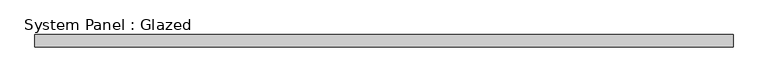
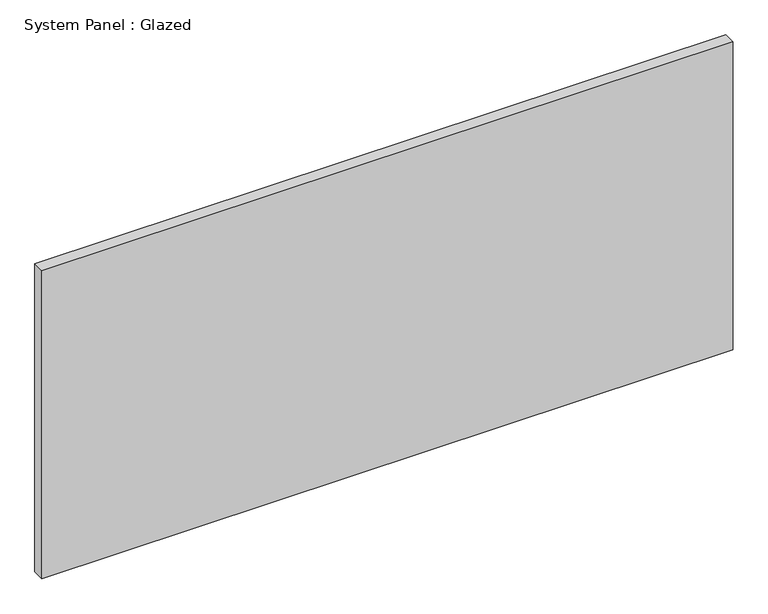
"""IFC4 building model written with IfcOpenShell, lengths in millimetres: plate geometry, System Panel : Glazed."""

from ifc_helpers import new_model, si_unit, origin, origin_with_axes, place, context, project, spatial, polyline, outline, extrude, source, transform, mapped, element, save


def system_panel_glazed_c279dccd(model_context):
    return source(origin(), model_context, "Body", "SweptSolid", [
        extrude(outline(polyline([(727.075, 19.05), (-727.075, 19.05), (-727.075, 44.45), (727.075, 44.45), (727.075, 19.05)])), origin_with_axes(), (0.0, 0.0, 1.0), 684.9785678),
    ])


if __name__ == "__main__":
    model = new_model("IFC4")
    model_context = context("Model", 3, world=origin())
    ifc_project = project(units=[si_unit("LENGTHUNIT", "METRE", prefix="MILLI")], contexts=[model_context])
    site = spatial("IfcSite", under=ifc_project)
    building = spatial("IfcBuilding", under=site)
    placement = place(None, origin())
    system_panel_glazed_shape = system_panel_glazed_c279dccd(model_context)
    element("IfcPlate", 1, ObjectType="System Panel : Glazed", at=placement, inside=building, context=model_context, shape_type="MappedRepresentation", body=[
        mapped(system_panel_glazed_shape, transform((0.0, 0.0, 0.0), x_axis=(1.0, 0.0, 0.0), y_axis=(0.0, 1.0, 0.0), z_axis=(0.0, 0.0, 1.0))),
    ])
    save(model, "model.ifc")

# Revit data of these elements
# Type "System Panel : Glazed"
#   Construction Type Id = "GSP4R"
#   Analytic Construction = "1/8 in Pilkington single glazing"
#   Visual Light Transmittance = 0.9
#   Solar Heat Gain Coefficient = 0.86
#   Heat Transfer Coefficient (U) = 1.18115 BTU/(h·ft²·°F)
#   Define Thermal Properties by = 1
# Element 1 (IfcPlate, "System Panel : Glazed")
#   Materials on its faces: "Glass"
# Materials
#   "Glass": class "Glass", colour RGB 0 128 192, transparency 0.75, Description = "Soda Lime Glass", Cost = 0
